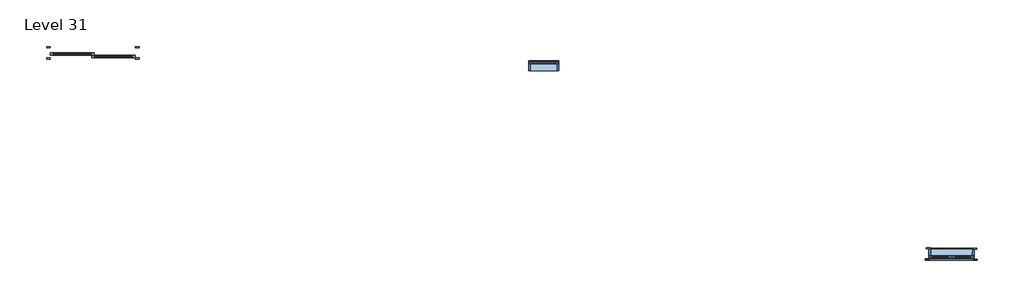
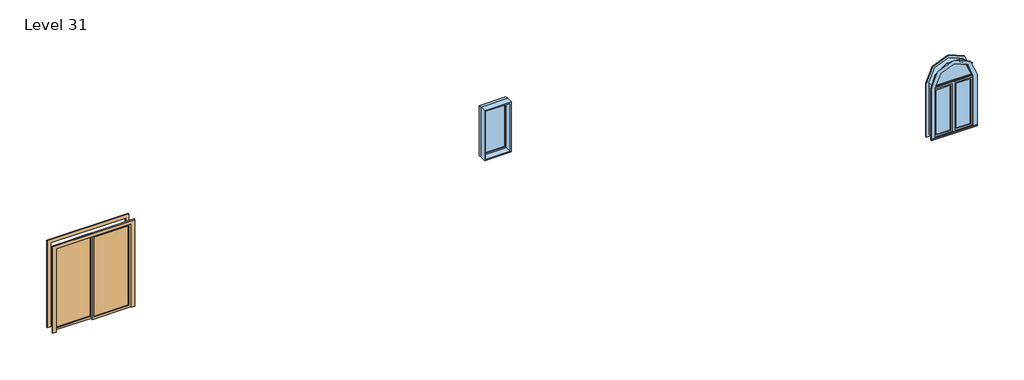
# One storey: 2 windows, 1 door.
"""IFC4 building model written with IfcOpenShell, lengths in millimetres."""

from ifc_helpers import new_model, si_unit, origin, place, context, project, spatial, transform, mapped, element, save
from components import door_076b30e0, window_cf4adaea, window_80bd9af0

model = new_model("IFC4")

# Units and contexts
model_context = context("Model", 3, world=origin())
ifc_project = project(units=[si_unit("LENGTHUNIT", "METRE", prefix="MILLI")], contexts=[model_context])

# Site, building, storey
site = spatial("IfcSite", under=ifc_project)
building = spatial("IfcBuilding", under=site)
storey = spatial("IfcBuildingStorey", under=building, Name="Level 31", Elevation=53035.2)

# Door
placement = place(None, origin())
door_shape = door_076b30e0(model_context)
element("IfcDoor", 1, ObjectType="Door-Double-Sliding : 68\" x 80\"", at=placement, inside=storey, context=model_context, shape_type="MappedRepresentation", body=[
    mapped(door_shape, transform((-16064.585279, -12227.7237084, 53035.2), x_axis=(-1.0, 0.0, 0.0), y_axis=(0.0, -1.0, 0.0), z_axis=(0.0, 0.0, 1.0))),
])

# Windows
window_shape = window_cf4adaea(model_context)
element("IfcWindow", 2, ObjectType="36\" x 48\"", at=placement, inside=storey, context=model_context, shape_type="MappedRepresentation", body=[
    mapped(window_shape, transform((1360.9377752, -16434.7461701, 53035.2), x_axis=(-0.9999808006467508, 0.006196639241010352, 0.0), y_axis=(-0.006196639241010352, -0.9999808006467508, 0.0), z_axis=(0.0, 0.0, 1.0))),
])
window_2_shape = window_80bd9af0(model_context)
element("IfcWindow", 3, ObjectType="Fixed : 24\" x 48\"", at=placement, inside=storey, context=model_context, shape_type="MappedRepresentation", body=[
    mapped(window_2_shape, transform((-6882.485279, -12617.2007309, 53035.2), x_axis=(1.0, 0.0, 0.0), y_axis=(0.0, 1.0, 0.0), z_axis=(0.0, 0.0, 1.0))),
])

save(model, "model.ifc")

# Revit data of these elements
# Type "Door-Double-Sliding : 68\" x 80\""
#   Type Mark = "10"
#   Construction Type Id = "opn-d45"
#   Assembly Code = "C1020"
#   Analytic Construction = "Wood frame, double glass door "
#   Thickness = 0' - 2"
#   Thermal Resistance (R) = 1.8150 (h·ft²·°F)/BTU
#   Heat Transfer Coefficient (U) = 0.5510 BTU/(h·ft²·°F)
#   Height = 6' - 8"
#   Rail Width = 0' - 2"
#   Stiles = 0' - 2"
#   Trim Projection Ext = 0' - 1"
#   Trim Projection Int = 0' - 1"
#   Trim Width = 0' - 3"
#   Width = 5' - 8"
#   Define Thermal Properties by = 1
#   Glazing = Glass
#   Panel Material = Wood - Birch - Solid Stained Light Low Gloss
#   Trim Material = Paint - Sienna
#   Visual Light Transmittance = 0
#   Solar Heat Gain Coefficient = 0
#   Function = (empty or 0)
#   Wall Closure = (empty or 0)
# Type "36\" x 48\""
#   Type Mark = "38"
#   Construction Type Id = "SGL"
#   Assembly Code = "B2020100"
#   Analytic Construction = "Large single-glazed windows"
#   Visual Light Transmittance = 0.9
#   Solar Heat Gain Coefficient = 0.86
#   Heat Transfer Coefficient (U) = 0.979472 BTU/(h·ft²·°F)
#   Height = 4' - 0"
#   Default Sill Height = 3' - 0"
#   Trim Projection - Ext. = 0' - 0 1/2"
#   Trim Projection - Int. = 0' - 0 3/4"
#   Trim Width - Exterior = 0' - 3 1/2"
#   Trim Width - Interior = 0' - 3 1/2"
#   Width = 3' - 0"
#   Window Inset = 0' - 0 3/4"
#   Define Thermal Properties by = 1
#   Glass Pane Material = Glass
#   Sash Material = Sash
#   Trim Exterior Material = Trim
#   Trim Interior Material = Trim
#   Wall Closure = (empty or 0)
# Type "Fixed : 24\" x 48\""
#   Type Mark = "2"
#   Construction Type Id = "GSP4R"
#   Assembly Code = "B2020100"
#   Analytic Construction = "1/8 in Pilkington single glazing"
#   Visual Light Transmittance = 0.9
#   Solar Heat Gain Coefficient = 0.78
#   Heat Transfer Coefficient (U) = 0.6496 BTU/(h·ft²·°F)
#   Height = 4' - 0"
#   Default Sill Height = 3' - 0"
#   Width = 2' - 0"
#   Window Inset = 0' - 0 3/4"
#   Define Thermal Properties by = 1
#   Glass Pane Material = Glass
#   Sash Material = Sash
#   Wall Closure = (empty or 0)
# Element 1 (IfcDoor, "Door-Double-Sliding : 68\" x 80\"")
#   Phase Created = New Construction
#   Materials on its faces: "Paint - Sienna", "Wood - Birch - Solid Stained Light Low Gloss", "Glass"
# Element 2 (IfcWindow, "36\" x 48\"")
#   Mark = "18"
#   Phase Created = New Construction
#   Materials on its faces: "Sash", "Trim", "Glass"
# Element 3 (IfcWindow, "Fixed : 24\" x 48\"")
#   Mark = "69"
#   Phase Created = New Construction
#   Materials on its faces: "Sash", "Glass"
# Materials
#   "Glass": class "Glass", colour RGB 0 128 192, transparency 0.75, Description = "Soda Lime Glass", Cost = 0
#   "Wood - Birch - Solid Stained Light Low Gloss": class "Wood", colour RGB 210 159 95, transparency 0, Cost = 0
#   "Paint - Sienna": colour RGB 118 70 51, transparency 0, Cost = 0
#   "Sash": class "Wood", colour RGB 224 178 126, transparency 0
#   "Trim": class "Wood", colour RGB 224 178 126, transparency 0
